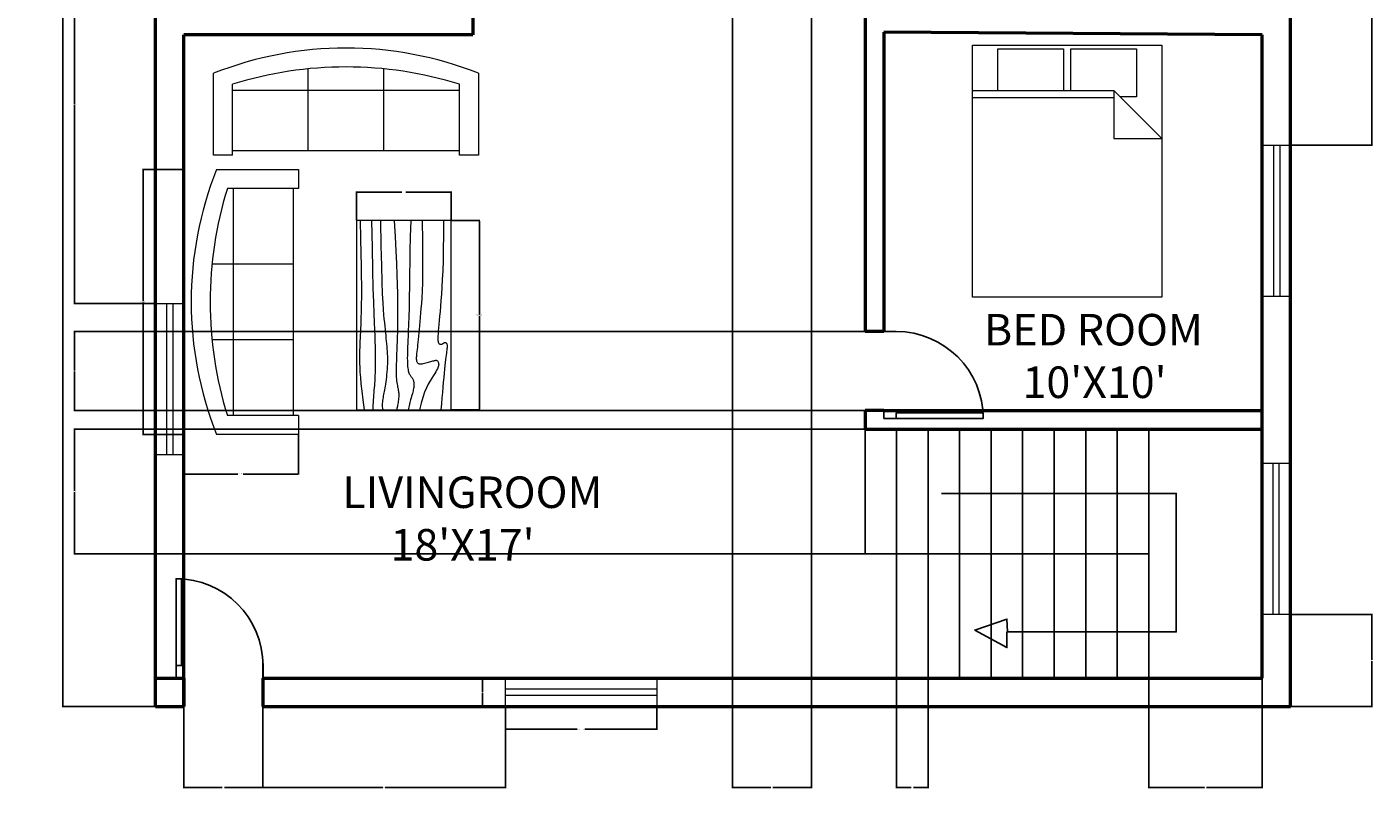
# Model space of a CAD drawing. Units: inches. Extents: x 471 to 898, y -3 to 533.
# Tile 1 of 3: x 471 to 898, y -3 to 239. Entities that reach past the tile are written whole.
import ezdxf

# ---------------------------------------------------------------- set-up
doc = ezdxf.new("R2010")
doc.units = ezdxf.units.IN
doc.header["$MEASUREMENT"] = 0
for name, color, linetype, lineweight in [('A-ANNO-DIMS', 2, 'Continuous', 18), ('A-AREA-IDEN', 7, 'Continuous', 25), ('A-DOOR', 3, 'Continuous', 25), ('A-FLOR-STRS', 7, 'Continuous', 25), ('A-FURN', 8, 'Continuous', 18), ('A-GLAZ', 4, 'Continuous', 18), ('A-WALL', 7, 'Continuous', 50)]:
    doc.layers.add(name, color=color, linetype=linetype, lineweight=lineweight)
doc.styles.get("Standard").update_dxf_attribs({"font": 'arial.ttf'})
doc.dimstyles.get("Standard").update_dxf_attribs({"dimtxt": 0.18, "dimasz": 0.18, "dimexe": 0.18, "dimexo": 0.0625, "dimgap": 0.09, "dimtad": 0, "dimtih": 1, "dimtoh": 1, "dimdec": 1, "dimzin": 0, "dimdsep": 46, "dimlunit": 4, "dimtxsty": 'Standard', "dimcen": 0.09, "dimadec": 0, "dimazin": 0, "dimtfac": 1, "dimtdec": 1, "dimtofl": 0, "dimtmove": 0, "dimatfit": 3, "dimfxl": 1, "dimtolj": 1, "dimtzin": 0, "dimarcsym": 0})

# ---------------------------------------------------------------- blocks, each defined once
blk = doc.blocks.new('Sofa - Roundback 7 ft.')
for p, q in [((-12.00002, -32.4421), (-12.00003, -6.5971)), ((11.99997, -32.4421), (11.99998, -6.5971)), ((-36.000027, -34), (-36.000027, -11.4696)), ((35.99998, -34), (35.99998, -11.4696)), ((-35.999844, -13.3819), (35.9998, -13.3819)), ((-36.000027, -32.4421), (35.99998, -32.4421))]:
    blk.add_line(p, q)
for points in [[(-36.000027, -34), (-42.000027, -34), (-42.000027, -8)], [(41.99998, -8), (41.99998, -34), (35.99998, -34)]]:
    blk.add_lwpolyline(points)
for centre, radius, start, end in [((0, -114.25), 114.25, 68.43141, 111.5686), ((-0.00001, -127.1968), 121.1968, 72.72033, 107.2797)]:
    blk.add_arc(centre, radius, start, end)
blk = doc.blocks.new('Table - Rectangular Woodgrain 60 x 30 in.')
for p, q in [((0, 0), (0, -30)), ((60, 0), (0, 0)), ((60, -30), (60, 0)), ((0, -30), (60, -30))]:
    blk.add_line(p, q)
for points in [[(0, -2.4), (4.8155, -2.418), (9.0302, -2.4688), (12.709, -2.5477), (15.9167, -2.65), (18.7181, -2.7711), (21.1781, -2.9063), (23.3616, -3.0508), (25.3333, -3.2), (27.1477, -3.3495), (28.8172, -3.4958), (30.3437, -3.636), (31.7291, -3.7667), (32.9756, -3.8849), (34.0849, -3.9875), (35.059, -4.0714), (35.9, -4.1334), (36.6114, -4.1711), (37.2041, -4.1854), (37.6906, -4.1779), (38.0833, -4.15), (38.3948, -4.1034), (38.6375, -4.0396), (38.8239, -3.9602), (38.9666, -3.8667), (39.0764, -3.7608), (39.1573, -3.6448), (39.2116, -3.521), (39.2416, -3.3917), (39.2498, -3.2593), (39.2385, -3.1261), (39.21, -2.9944), (39.1666, -2.8667), (39.111, -2.7447), (39.0468, -2.6281), (38.978, -2.5163), (38.9083, -2.4083), (38.8418, -2.3035), (38.7823, -2.201), (38.7337, -2.1001), (38.7, -2), (38.6844, -1.9003), (38.6875, -1.8021), (38.7094, -1.707), (38.75, -1.6167), (38.8094, -1.5326), (38.8875, -1.4563), (38.9844, -1.3893), (39.1, -1.3333), (39.2351, -1.2896), (39.3937, -1.2583), (39.5804, -1.2396), (39.8, -1.2333), (40.057, -1.2396), (40.3562, -1.2583), (40.7023, -1.2896), (41.1, -1.3333), (41.5547, -1.3895), (42.0755, -1.4573), (42.6721, -1.5361), (43.3542, -1.625), (44.1316, -1.7233), (45.014, -1.8302), (46.0114, -1.9449), (47.1333, -2.0667), (48.3862, -2.1947), (49.7625, -2.3281), (51.2513, -2.4663), (52.8416, -2.6083), (54.5226, -2.7535), (56.2833, -2.9011), (58.1127, -3.0501), (60, -3.2)], [(0, -9.2), (6.5759, -9.0858), (11.9385, -9.0365), (16.2527, -9.0418), (19.6833, -9.0917), (22.3952, -9.1759), (24.5531, -9.2844), (26.322, -9.4069), (27.8666, -9.5333), (29.3241, -9.6553), (30.7203, -9.7719), (32.0532, -9.8837), (33.3208, -9.9917), (34.5213, -10.0965), (35.6526, -10.199), (36.7128, -10.2999), (37.7, -10.4), (38.6129, -10.4996), (39.4531, -10.5969), (40.223, -10.6895), (40.925, -10.775), (41.5613, -10.8512), (42.1344, -10.9156), (42.6465, -10.966), (43.1, -11), (43.4976, -11.0158), (43.8437, -11.0136), (44.143, -10.9942), (44.4, -10.9583), (44.6195, -10.9069), (44.8062, -10.8406), (44.9648, -10.7603), (45.1, -10.6667), (45.2155, -10.5598), (45.3114, -10.4365), (45.3871, -10.2929), (45.4416, -10.125), (45.4743, -9.929), (45.4844, -9.7011), (45.4709, -9.4371), (45.4333, -9.1333), (45.3716, -8.7883), (45.2896, -8.4104), (45.1919, -8.0107), (45.0833, -7.6), (44.9685, -7.1893), (44.8521, -6.7896), (44.7388, -6.4117), (44.6333, -6.0667), (44.54, -5.7628), (44.4614, -5.4979), (44.4001, -5.2675), (44.3583, -5.0667), (44.3384, -4.8909), (44.3427, -4.7354), (44.3736, -4.5956), (44.4333, -4.4667), (44.5236, -4.3453), (44.6427, -4.2333), (44.7884, -4.1339), (44.9583, -4.05), (45.1501, -3.9849), (45.3614, -3.9417), (45.59, -3.9234), (45.8333, -3.9333), (46.0915, -3.9749), (46.3734, -4.0531), (46.6906, -4.1736), (47.0542, -4.3417), (47.4756, -4.5629), (47.9661, -4.8427), (48.5372, -5.1866), (49.2, -5.6), (49.9676, -6.0844), (50.8594, -6.625), (51.8965, -7.2031), (53.1, -7.8), (54.491, -8.3969), (56.0906, -8.975), (57.9199, -9.5156), (60, -10)], [(0, -12.8), (5.1847, -12.9322), (9.6213, -13.0323), (13.3963, -13.1059), (16.5958, -13.1583), (19.3063, -13.1952), (21.614, -13.2219), (23.6054, -13.2439), (25.3666, -13.2667), (26.9728, -13.2947), (28.4531, -13.3281), (29.8256, -13.3663), (31.1083, -13.4083), (32.3191, -13.4535), (33.476, -13.501), (34.597, -13.5501), (35.7, -13.6), (36.7984, -13.6497), (37.8875, -13.6979), (38.9578, -13.743), (40, -13.7833), (41.0047, -13.8174), (41.9625, -13.8438), (42.864, -13.8607), (43.7, -13.8667), (44.4631, -13.8604), (45.1552, -13.8417), (45.7801, -13.8104), (46.3416, -13.7667), (46.8439, -13.7104), (47.2906, -13.6417), (47.6858, -13.5604), (48.0333, -13.4667), (48.3375, -13.3608), (48.6042, -13.2448), (48.8396, -13.121), (49.05, -12.9917), (49.2417, -12.8593), (49.4208, -12.7261), (49.5937, -12.5944), (49.7667, -12.4667), (49.9452, -12.3451), (50.1323, -12.2313), (50.3303, -12.1268), (50.5416, -12.0333), (50.7686, -11.9524), (51.0135, -11.8854), (51.2788, -11.8341), (51.5666, -11.8), (51.8785, -11.7843), (52.2116, -11.7865), (52.562, -11.8059), (52.926, -11.8417), (53.2998, -11.8931), (53.6795, -11.9594), (54.0614, -12.0397), (54.4416, -12.1333), (54.8223, -12.2401), (55.2293, -12.3625), (55.6942, -12.5037), (56.2489, -12.6667), (56.9251, -12.8547), (57.7545, -13.0708), (58.7689, -13.3182), (60, -13.6)], [(0, -18), (5.124, -17.7273), (9.6609, -17.5057), (13.6705, -17.3303), (17.2125, -17.1958), (20.3467, -17.0973), (23.1328, -17.0297), (25.6307, -16.9878), (27.9, -16.9667), (29.9928, -16.9617), (31.9302, -16.9703), (33.7254, -16.9907), (35.3917, -17.0208), (36.9423, -17.0588), (38.3906, -17.1026), (39.7499, -17.1503), (41.0333, -17.2), (42.2519, -17.2496), (43.4073, -17.2969), (44.4986, -17.3395), (45.525, -17.375), (46.4858, -17.4012), (47.3802, -17.4156), (48.2074, -17.416), (48.9667, -17.4), (49.6583, -17.3662), (50.2872, -17.3167), (50.8595, -17.2547), (51.3812, -17.1833), (51.8584, -17.1057), (52.2971, -17.025), (52.7034, -16.9443), (53.0833, -16.8667), (53.443, -16.7951), (53.789, -16.7313), (54.128, -16.6768), (54.4666, -16.6334), (54.8115, -16.6024), (55.1693, -16.5854), (55.5465, -16.5841), (55.95, -16.6), (56.3828, -16.6337), (56.8346, -16.6823), (57.2915, -16.7418), (57.7396, -16.8084), (58.165, -16.878), (58.5539, -16.9469), (58.8924, -17.0111), (59.1666, -17.0667), (59.3679, -17.1107), (59.5078, -17.1438), (59.6032, -17.1675), (59.6708, -17.1833), (59.7275, -17.193), (59.7901, -17.1979), (59.8753, -17.1998), (60, -17.2)], [(0, -22.4), (8.0098, -22.2501), (14.4094, -22.1011), (19.4168, -21.9535), (23.25, -21.8083), (26.1269, -21.6663), (28.2656, -21.5281), (29.884, -21.3947), (31.2, -21.2667), (32.3967, -21.1448), (33.5172, -21.0292), (34.5697, -20.9198), (35.5625, -20.8167), (36.5037, -20.7198), (37.4015, -20.6292), (38.2642, -20.5448), (39.1, -20.4667), (39.9164, -20.3951), (40.7187, -20.3313), (41.5117, -20.2768), (42.3, -20.2333), (43.0883, -20.2024), (43.8812, -20.1854), (44.6836, -20.1841), (45.5, -20.2), (46.3328, -20.234), (47.1747, -20.2844), (48.0163, -20.3488), (48.8479, -20.425), (49.66, -20.5106), (50.4429, -20.6031), (51.1872, -20.7004), (51.8833, -20.8), (52.5246, -20.8999), (53.1166, -20.9995), (53.6681, -21.0983), (54.1875, -21.1958), (54.6834, -21.2919), (55.1646, -21.3859), (55.6394, -21.4777), (56.1167, -21.5667), (56.6028, -21.6515), (57.0961, -21.7266), (57.5929, -21.7852), (58.0896, -21.8208), (58.5823, -21.8268), (59.0674, -21.7964), (59.5412, -21.723), (60, -21.6)], [(0, -25.2), (8.6355, -25.0504), (15.7026, -24.9031), (21.4049, -24.7606), (25.9458, -24.625), (29.529, -24.4988), (32.3578, -24.3844), (34.6359, -24.284), (36.5667, -24.2), (38.3213, -24.1341), (39.9417, -24.0854), (41.437, -24.0523), (42.8167, -24.0333), (44.0901, -24.0268), (45.2667, -24.0313), (46.3557, -24.0451), (47.3667, -24.0667), (48.309, -24.0947), (49.1928, -24.1287), (50.0284, -24.168), (50.826, -24.2125), (51.5959, -24.2617), (52.3483, -24.3151), (53.0935, -24.3725), (53.8417, -24.4334), (54.6009, -24.497), (55.3699, -24.561), (56.1454, -24.6226), (56.9239, -24.6792), (57.7021, -24.7279), (58.4764, -24.7662), (59.2435, -24.7911), (60, -24.8)], [(0, -28.8), (5.6867, -28.6681), (10.45, -28.5698), (14.407, -28.5012), (17.675, -28.4584), (20.3711, -28.4374), (22.6125, -28.4344), (24.5164, -28.4455), (26.2, -28.4667), (27.762, -28.4947), (29.2276, -28.5281), (30.6033, -28.5663), (31.8958, -28.6084), (33.1118, -28.6535), (34.2578, -28.7011), (35.3405, -28.7501), (36.3666, -28.8), (37.3443, -28.8497), (38.288, -28.8974), (39.2137, -28.9412), (40.1375, -28.9792), (41.0753, -29.0093), (42.0432, -29.0297), (43.0572, -29.0384), (44.1333, -29.0333), (45.2936, -29.0114), (46.5843, -28.9641), (48.0579, -28.8816), (49.7666, -28.7542), (51.7629, -28.5721), (54.0989, -28.3255), (56.8272, -28.0048), (60, -27.6)]]:
    blk.add_lwpolyline(points)
blk = doc.blocks.new('Bed - Queen')
for p, q in [((0, -80.00003), (0, 0)), ((0, 0), (59.99999, 0)), ((59.99999, 0), (59.99999, -80.00003)), ((7.99999, -1.2), (28.79998, -1.2)), ((7.99999, -14.4), (7.99999, -1.2)), ((28.79998, -1.2), (28.79998, -14.4)), ((31.19999, -1.2), (51.99999, -1.2)), ((31.19999, -14.4), (31.19999, -1.2)), ((51.99999, -1.2), (51.99999, -16.4)), ((0, -14.4), (44.8, -14.4)), ((44.8, -16.8), (0, -16.8)), ((59.99999, -29.6), (44.8, -14.4)), ((44.8, -14.4), (44.8, -29.6)), ((51.99999, -16.4), (46.79936, -16.4)), ((44.8, -29.6), (59.99999, -29.6)), ((59.99999, -80.00003), (0, -80.00003))]:
    blk.add_line(p, q)
blk = doc.blocks.new('*U8')
for p, q in [((0, 0), (0, -100)), ((700, 0), (700, -100))]:
    blk.add_line(p, q)
blk.add_lwpolyline([(0, 0), (0, 700), (43.75, 700), (43.75, 0)], close=True)
blk.add_arc((0, 0), 700, 0, 90)
blk = doc.blocks.new('*D13')
at = {"layer": 'A-ANNO-DIMS', "color": 0, "lineweight": -2, "transparency": 16777216}
for p, q in [((512.17, 503.07), (482.62, 503.07)), ((482.8, 502.89), (482.8, 269.29)), ((482.8, 23.25), (482.8, 256.86)), ((512.17, 23.07), (482.62, 23.07))]:
    blk.add_line(p, q, dxfattribs=at)
at = {"layer": 'A-ANNO-DIMS', "color": 0, "transparency": 16777216}
for points in [[(482.77, 502.89), (482.83, 502.89), (482.8, 503.07)], [(482.77, 23.25), (482.83, 23.25), (482.8, 23.07)]]:
    blk.add_solid(points, dxfattribs=at)
at = {"layer": 'Defpoints', "color": 0, "transparency": 16777216}
for p in [(512.23, 503.07), (482.8, 23.07), (512.23, 23.07)]:
    blk.add_point(p, dxfattribs=at)
at = {"layer": 'A-ANNO-DIMS', "color": 0, "transparency": 16777216, "insert": (482.8, 263.07), "char_height": 12, "attachment_point": 5}
blk.add_mtext("\\A1;40'", dxfattribs=at)
blk = doc.blocks.new('WIN-48X9')
for p, q in [((0, 48), (9, 48)), ((0, 0), (0, 48)), ((3.5, 48), (3.5, 0)), ((5.5, 48), (5.5, 0)), ((9, 48), (9, 0)), ((9, 0), (0, 0))]:
    blk.add_line(p, q)
blk = doc.blocks.new('*D15')
at = {"layer": 'A-ANNO-DIMS', "color": 0, "lineweight": -2, "transparency": 16777216}
for p, q in [((623.17, 23.01), (623.17, 15.69)), ((671.17, 23.01), (671.17, 15.69)), ((623.35, 15.87), (645.94, 15.87)), ((670.99, 15.87), (648.4, 15.87))]:
    blk.add_line(p, q, dxfattribs=at)
at = {"layer": 'A-ANNO-DIMS', "color": 0, "transparency": 16777216}
for points in [[(623.35, 15.9), (623.35, 15.84), (623.17, 15.87)], [(670.99, 15.9), (670.99, 15.84), (671.17, 15.87)]]:
    blk.add_solid(points, dxfattribs=at)
at = {"layer": 'Defpoints', "color": 0, "transparency": 16777216}
for p in [(623.17, 23.07), (671.17, 23.07), (671.17, 15.87)]:
    blk.add_point(p, dxfattribs=at)
at = {"layer": 'A-ANNO-DIMS', "color": 0, "transparency": 16777216, "insert": (647.17, 15.87), "char_height": 0.18, "attachment_point": 5}
blk.add_mtext('\\A1;WINDOW 4\'-0" TYP.', dxfattribs=at)
blk = doc.blocks.new('*D16')
at = {"layer": 'A-ANNO-DIMS', "color": 0, "lineweight": -2, "transparency": 16777216}
for p, q in [((623.11, 32.07), (615.79, 32.07)), ((615.97, 31.89), (615.97, 27.76)), ((615.97, 23.25), (615.97, 27.39)), ((623.11, 23.07), (615.79, 23.07))]:
    blk.add_line(p, q, dxfattribs=at)
at = {"layer": 'A-ANNO-DIMS', "color": 0, "transparency": 16777216}
for points in [[(615.94, 31.89), (616, 31.89), (615.97, 32.07)], [(615.94, 23.25), (616, 23.25), (615.97, 23.07)]]:
    blk.add_solid(points, dxfattribs=at)
at = {"layer": 'Defpoints', "color": 0, "transparency": 16777216}
for p in [(623.17, 32.07), (615.97, 23.07), (623.17, 23.07)]:
    blk.add_point(p, dxfattribs=at)
at = {"layer": 'A-ANNO-DIMS', "color": 0, "transparency": 16777216, "insert": (615.97, 27.57), "char_height": 0.18, "attachment_point": 5}
blk.add_mtext('\\A1;0\'-9" TYP.', dxfattribs=at)
blk = doc.blocks.new('*D19')
at = {"layer": 'A-ANNO-DIMS', "color": 0, "lineweight": -2, "transparency": 16777216}
for p, q in [((606.01, 177.21), (615.13, 177.21)), ((614.95, 177.03), (614.95, 147.39)), ((614.95, 117.39), (614.95, 147.03)), ((606.01, 117.21), (615.13, 117.21))]:
    blk.add_line(p, q, dxfattribs=at)
at = {"layer": 'A-ANNO-DIMS', "color": 0, "transparency": 16777216}
for points in [[(614.92, 177.03), (614.98, 177.03), (614.95, 177.21)], [(614.92, 117.39), (614.98, 117.39), (614.95, 117.21)]]:
    blk.add_solid(points, dxfattribs=at)
at = {"layer": 'Defpoints', "color": 0, "transparency": 16777216}
for p in [(605.95, 177.21), (605.95, 117.21), (614.95, 117.21)]:
    blk.add_point(p, dxfattribs=at)
at = {"layer": 'A-ANNO-DIMS', "color": 0, "transparency": 16777216, "insert": (614.95, 147.21), "char_height": 0.18, "attachment_point": 5}
blk.add_mtext('\\A1;TABLE 5\'-0" TYP.', dxfattribs=at)
blk = doc.blocks.new('*D20')
at = {"layer": 'A-ANNO-DIMS', "color": 0, "lineweight": -2, "transparency": 16777216}
for p, q in [((575.95, 177.28), (575.95, 186.39)), ((576.13, 186.21), (590.31, 186.21)), ((605.77, 186.21), (591.59, 186.21)), ((605.95, 177.28), (605.95, 186.39))]:
    blk.add_line(p, q, dxfattribs=at)
at = {"layer": 'A-ANNO-DIMS', "color": 0, "transparency": 16777216}
for points in [[(576.13, 186.24), (576.13, 186.18), (575.95, 186.21)], [(605.77, 186.24), (605.77, 186.18), (605.95, 186.21)]]:
    blk.add_solid(points, dxfattribs=at)
at = {"layer": 'Defpoints', "color": 0, "transparency": 16777216}
for p in [(605.95, 186.21), (575.95, 177.21), (605.95, 177.21)]:
    blk.add_point(p, dxfattribs=at)
at = {"layer": 'A-ANNO-DIMS', "color": 0, "transparency": 16777216, "insert": (590.95, 186.21), "char_height": 0.18, "attachment_point": 5}
blk.add_mtext('\\A1;2\'-6" TYP.', dxfattribs=at)
blk = doc.blocks.new('*D21')
at = {"layer": 'A-ANNO-DIMS', "color": 0, "lineweight": -2, "transparency": 16777216}
for p, q in [((520.81, 193.39), (508.09, 193.39)), ((508.27, 193.21), (508.27, 151.58)), ((508.27, 109.57), (508.27, 151.21)), ((520.81, 109.39), (508.09, 109.39))]:
    blk.add_line(p, q, dxfattribs=at)
at = {"layer": 'A-ANNO-DIMS', "color": 0, "transparency": 16777216}
for points in [[(508.24, 193.21), (508.3, 193.21), (508.27, 193.39)], [(508.24, 109.57), (508.3, 109.57), (508.27, 109.39)]]:
    blk.add_solid(points, dxfattribs=at)
at = {"layer": 'Defpoints', "color": 0, "transparency": 16777216}
for p in [(508.27, 193.39), (520.87, 193.39), (520.87, 109.39)]:
    blk.add_point(p, dxfattribs=at)
at = {"layer": 'A-ANNO-DIMS', "color": 0, "transparency": 16777216, "insert": (508.27, 151.39), "char_height": 0.18, "attachment_point": 5}
blk.add_mtext('\\A1;SOFA 7\'-0" TYP.', dxfattribs=at)
blk = doc.blocks.new('*D22')
at = {"layer": 'A-ANNO-DIMS', "color": 0, "lineweight": -2, "transparency": 16777216}
for p, q in [((520.87, 109.33), (520.87, 96.61)), ((557.54, 109.33), (557.54, 96.61)), ((521.05, 96.79), (538.36, 96.79)), ((557.36, 96.79), (540.05, 96.79))]:
    blk.add_line(p, q, dxfattribs=at)
at = {"layer": 'A-ANNO-DIMS', "color": 0, "transparency": 16777216}
for points in [[(521.05, 96.82), (521.05, 96.76), (520.87, 96.79)], [(557.36, 96.82), (557.36, 96.76), (557.54, 96.79)]]:
    blk.add_solid(points, dxfattribs=at)
at = {"layer": 'Defpoints', "color": 0, "transparency": 16777216}
for p in [(520.87, 109.39), (557.54, 109.39), (520.87, 96.79)]:
    blk.add_point(p, dxfattribs=at)
at = {"layer": 'A-ANNO-DIMS', "color": 0, "transparency": 16777216, "insert": (539.21, 96.79), "char_height": 0.18, "attachment_point": 5}
blk.add_mtext('\\A1;3\'-0 1/2" TYP.', dxfattribs=at)
blk = doc.blocks.new('*D33')
at = {"layer": 'A-ANNO-DIMS', "color": 0, "lineweight": -2, "transparency": 16777216}
for p, q in [((521.23, 23.01), (521.23, -2.81)), ((546.23, 23.01), (546.23, -2.81)), ((521.41, -2.63), (533.4, -2.63)), ((546.05, -2.63), (534.06, -2.63))]:
    blk.add_line(p, q, dxfattribs=at)
at = {"layer": 'A-ANNO-DIMS', "color": 0, "transparency": 16777216}
for points in [[(521.41, -2.6), (521.41, -2.66), (521.23, -2.63)], [(546.05, -2.6), (546.05, -2.66), (546.23, -2.63)]]:
    blk.add_solid(points, dxfattribs=at)
at = {"layer": 'Defpoints', "color": 0, "transparency": 16777216}
for p in [(521.23, 23.07), (546.23, 23.07), (546.23, -2.63)]:
    blk.add_point(p, dxfattribs=at)
at = {"layer": 'A-ANNO-DIMS', "color": 0, "transparency": 16777216, "insert": (533.73, -2.63), "char_height": 0.18, "attachment_point": 5}
blk.add_mtext('\\A1;2\'-1"', dxfattribs=at)
blk = doc.blocks.new('*D34')
at = {"layer": 'A-ANNO-DIMS', "color": 0, "lineweight": -2, "transparency": 16777216}
for p, q in [((546.23, 23.01), (546.23, -2.81)), ((623.17, 23.01), (623.17, -2.81)), ((546.41, -2.63), (584.37, -2.63)), ((622.99, -2.63), (585.03, -2.63))]:
    blk.add_line(p, q, dxfattribs=at)
at = {"layer": 'A-ANNO-DIMS', "color": 0, "transparency": 16777216}
for points in [[(546.41, -2.6), (546.41, -2.66), (546.23, -2.63)], [(622.99, -2.6), (622.99, -2.66), (623.17, -2.63)]]:
    blk.add_solid(points, dxfattribs=at)
at = {"layer": 'Defpoints', "color": 0, "transparency": 16777216}
for p in [(546.23, 23.07), (623.17, 23.07), (623.17, -2.63)]:
    blk.add_point(p, dxfattribs=at)
at = {"layer": 'A-ANNO-DIMS', "color": 0, "transparency": 16777216, "insert": (584.7, -2.63), "char_height": 0.18, "attachment_point": 5}
blk.add_mtext('\\A1;6\'-5"', dxfattribs=at)
blk = doc.blocks.new('*D37')
at = {"layer": 'A-ANNO-DIMS', "color": 0, "lineweight": -2, "transparency": 16777216}
for p, q in [((512.17, 277.18), (486.35, 277.18)), ((486.53, 277), (486.53, 214.23)), ((486.53, 151.09), (486.53, 213.86)), ((512.17, 150.91), (486.35, 150.91))]:
    blk.add_line(p, q, dxfattribs=at)
at = {"layer": 'A-ANNO-DIMS', "color": 0, "transparency": 16777216}
for points in [[(486.5, 277), (486.56, 277), (486.53, 277.18)], [(486.5, 151.09), (486.56, 151.09), (486.53, 150.91)]]:
    blk.add_solid(points, dxfattribs=at)
at = {"layer": 'Defpoints', "color": 0, "transparency": 16777216}
for p in [(512.23, 277.18), (486.53, 150.91), (512.23, 150.91)]:
    blk.add_point(p, dxfattribs=at)
at = {"layer": 'A-ANNO-DIMS', "color": 0, "transparency": 16777216, "insert": (486.53, 214.04), "char_height": 0.18, "attachment_point": 5}
blk.add_mtext('\\A1;10\'-6 1/2"', dxfattribs=at)
blk = doc.blocks.new('*D40')
at = {"layer": 'A-ANNO-DIMS', "color": 0, "lineweight": -2, "transparency": 16777216}
for p, q in [((872.29, 380.09), (898.15, 380.09)), ((897.97, 379.91), (897.97, 290.77)), ((897.97, 201.27), (897.97, 290.41)), ((872.33, 201.09), (898.15, 201.09))]:
    blk.add_line(p, q, dxfattribs=at)
at = {"layer": 'A-ANNO-DIMS', "color": 0, "transparency": 16777216}
for points in [[(897.94, 379.91), (898, 379.91), (897.97, 380.09)], [(897.94, 201.27), (898, 201.27), (897.97, 201.09)]]:
    blk.add_solid(points, dxfattribs=at)
at = {"layer": 'Defpoints', "color": 0, "transparency": 16777216}
for p in [(872.23, 380.09), (872.27, 201.09), (897.97, 201.09)]:
    blk.add_point(p, dxfattribs=at)
at = {"layer": 'A-ANNO-DIMS', "color": 0, "transparency": 16777216, "insert": (897.97, 290.59), "char_height": 0.18, "attachment_point": 5}
blk.add_mtext('\\A1;14\'-11"', dxfattribs=at)
blk = doc.blocks.new('*D41')
at = {"layer": 'A-ANNO-DIMS', "color": 0, "lineweight": -2, "transparency": 16777216}
for p, q in [((872.1, 52.21), (898.15, 52.21)), ((897.97, 52.03), (897.97, 37.83)), ((897.97, 23.25), (897.97, 37.46)), ((872.29, 23.07), (898.15, 23.07))]:
    blk.add_line(p, q, dxfattribs=at)
at = {"layer": 'A-ANNO-DIMS', "color": 0, "transparency": 16777216}
for points in [[(897.94, 52.03), (898, 52.03), (897.97, 52.21)], [(897.94, 23.25), (898, 23.25), (897.97, 23.07)]]:
    blk.add_solid(points, dxfattribs=at)
at = {"layer": 'Defpoints', "color": 0, "transparency": 16777216}
for p in [(872.04, 52.21), (897.97, 52.21), (872.23, 23.07)]:
    blk.add_point(p, dxfattribs=at)
at = {"layer": 'A-ANNO-DIMS', "color": 0, "transparency": 16777216, "insert": (897.97, 37.64), "char_height": 0.18, "attachment_point": 5}
blk.add_mtext('\\A1;2\'-5"', dxfattribs=at)
blk = doc.blocks.new('*D42')
at = {"layer": 'A-ANNO-DIMS', "color": 0, "lineweight": -2, "transparency": 16777216}
for p, q in [((737.17, 111), (486.35, 111)), ((486.53, 110.82), (486.53, 91.45)), ((486.53, 71.72), (486.53, 91.09)), ((737.17, 71.54), (486.35, 71.54))]:
    blk.add_line(p, q, dxfattribs=at)
at = {"layer": 'A-ANNO-DIMS', "color": 0, "transparency": 16777216}
for points in [[(486.5, 110.82), (486.56, 110.82), (486.53, 111)], [(486.5, 71.72), (486.56, 71.72), (486.53, 71.54)]]:
    blk.add_solid(points, dxfattribs=at)
at = {"layer": 'Defpoints', "color": 0, "transparency": 16777216}
for p in [(486.53, 111), (737.24, 111), (737.24, 71.54)]:
    blk.add_point(p, dxfattribs=at)
at = {"layer": 'A-ANNO-DIMS', "color": 0, "transparency": 16777216, "insert": (486.53, 91.27), "char_height": 0.18, "attachment_point": 5}
blk.add_mtext('\\A1;3\'-3 1/2"', dxfattribs=at)
blk = doc.blocks.new('*D43')
at = {"layer": 'A-ANNO-DIMS', "color": 0, "lineweight": -2, "transparency": 16777216}
for p, q in [((827.24, 32.01), (827.24, -2.81)), ((863.23, 32.01), (863.23, -2.81)), ((827.42, -2.63), (844.9, -2.63)), ((863.05, -2.63), (845.56, -2.63))]:
    blk.add_line(p, q, dxfattribs=at)
at = {"layer": 'A-ANNO-DIMS', "color": 0, "transparency": 16777216}
for points in [[(827.42, -2.6), (827.42, -2.66), (827.24, -2.63)], [(863.05, -2.6), (863.05, -2.66), (863.23, -2.63)]]:
    blk.add_solid(points, dxfattribs=at)
at = {"layer": 'Defpoints', "color": 0, "transparency": 16777216}
for p in [(827.24, 32.07), (863.23, 32.07), (863.23, -2.63)]:
    blk.add_point(p, dxfattribs=at)
at = {"layer": 'A-ANNO-DIMS', "color": 0, "transparency": 16777216, "insert": (845.23, -2.63), "char_height": 0.18, "attachment_point": 5}
blk.add_mtext('\\A1;3\'-0"', dxfattribs=at)
blk = doc.blocks.new('*D46')
at = {"layer": 'A-ANNO-DIMS', "color": 0, "lineweight": -2, "transparency": 16777216}
for p, q in [((747.24, 32.01), (747.24, -2.81)), ((757.24, 32.01), (757.24, -2.81)), ((747.42, -2.63), (751.84, -2.63)), ((757.06, -2.63), (752.63, -2.63))]:
    blk.add_line(p, q, dxfattribs=at)
at = {"layer": 'A-ANNO-DIMS', "color": 0, "transparency": 16777216}
for points in [[(747.42, -2.6), (747.42, -2.66), (747.24, -2.63)], [(757.06, -2.6), (757.06, -2.66), (757.24, -2.63)]]:
    blk.add_solid(points, dxfattribs=at)
at = {"layer": 'Defpoints', "color": 0, "transparency": 16777216}
for p in [(747.24, 32.07), (757.24, 32.07), (757.24, -2.63)]:
    blk.add_point(p, dxfattribs=at)
at = {"layer": 'A-ANNO-DIMS', "color": 0, "transparency": 16777216, "insert": (752.24, -2.63), "char_height": 0.18, "attachment_point": 5}
blk.add_mtext('\\A1;0\'-10"', dxfattribs=at)
blk = doc.blocks.new('*D48')
at = {"layer": 'A-ANNO-DIMS', "color": 0, "lineweight": -2, "transparency": 16777216}
for p, q in [((695.23, 314.01), (695.23, -2.81)), ((720.23, 314.01), (720.23, -2.81)), ((695.41, -2.63), (707.4, -2.63)), ((720.05, -2.63), (708.06, -2.63))]:
    blk.add_line(p, q, dxfattribs=at)
at = {"layer": 'A-ANNO-DIMS', "color": 0, "transparency": 16777216}
for points in [[(695.41, -2.6), (695.41, -2.66), (695.23, -2.63)], [(720.05, -2.6), (720.05, -2.66), (720.23, -2.63)]]:
    blk.add_solid(points, dxfattribs=at)
at = {"layer": 'Defpoints', "color": 0, "transparency": 16777216}
for p in [(695.23, 314.07), (720.23, 314.07), (720.23, -2.63)]:
    blk.add_point(p, dxfattribs=at)
at = {"layer": 'A-ANNO-DIMS', "color": 0, "transparency": 16777216, "insert": (707.73, -2.63), "char_height": 0.18, "attachment_point": 5}
blk.add_mtext('\\A1;2\'-1"', dxfattribs=at)
blk = doc.blocks.new('*D49')
at = {"layer": 'A-ANNO-DIMS', "color": 0, "lineweight": -2, "transparency": 16777216}
for p, q in [((737.17, 142), (486.35, 142)), ((486.53, 141.82), (486.53, 129.68)), ((486.53, 117.18), (486.53, 129.32)), ((737.17, 117), (486.35, 117))]:
    blk.add_line(p, q, dxfattribs=at)
at = {"layer": 'A-ANNO-DIMS', "color": 0, "transparency": 16777216}
for points in [[(486.5, 141.82), (486.56, 141.82), (486.53, 142)], [(486.5, 117.18), (486.56, 117.18), (486.53, 117)]]:
    blk.add_solid(points, dxfattribs=at)
at = {"layer": 'Defpoints', "color": 0, "transparency": 16777216}
for p in [(486.53, 142), (737.24, 142), (737.24, 117)]:
    blk.add_point(p, dxfattribs=at)
at = {"layer": 'A-ANNO-DIMS', "color": 0, "transparency": 16777216, "insert": (486.53, 129.5), "char_height": 0.18, "attachment_point": 5}
blk.add_mtext('\\A1;2\'-1"', dxfattribs=at)

msp = doc.modelspace()

# ---------------------------------------------------------------- linework, layer by layer
at = {"layer": 'A-DOOR'}
for p, q in [((743.24, 117.21), (743.24, 117)), ((743.24, 114.44), (743.24, 117)), ((521.23, 38.07), (521.23, 32.07)), ((546.23, 38.07), (546.23, 32.07)), ((518.76, 32.12), (521.23, 32.07))]:
    msp.add_line(p, q, dxfattribs=at)
at = {"layer": 'A-FLOR-STRS'}
for p, q in [((737.24, 111), (737.24, 71.54)), ((747.24, 111), (747.24, 32.07)), ((757.24, 111), (757.24, 32.07)), ((767.24, 111), (767.24, 32.07)), ((777.24, 111), (777.24, 32.07)), ((787.24, 111), (787.24, 32.07)), ((797.24, 111), (797.24, 32.07)), ((807.24, 111), (807.24, 32.07)), ((817.24, 111), (817.24, 32.07)), ((827.24, 111), (827.24, 32.07)), ((737.24, 71.54), (827.24, 71.54))]:
    msp.add_line(p, q, dxfattribs=at)
msp.add_lwpolyline([(761.52, 90.66), (835.95, 90.66), (835.95, 46.7), (782.23, 46.7), (782.23, 41.74), (772.04, 47.32), (782.24, 50.82), (782.4, 46.7)], dxfattribs=at)
at = {"layer": 'A-WALL'}
for p, q in [((512.23, 23.07), (512.23, 503.07)), ((872.23, 23.07), (872.23, 503.07)), ((612.83, 242.07), (612.83, 236.07)), ((737.24, 243.05), (737.24, 142)), ((521.23, 23.07), (521.23, 236.07)), ((612.83, 236.07), (521.23, 236.07)), ((863.23, 236.07), (743.24, 237)), ((743.24, 237), (743.24, 142)), ((863.23, 32.07), (863.23, 236.07)), ((743.24, 142), (737.24, 142)), ((743.24, 117), (737.24, 117)), ((737.24, 117), (737.24, 111)), ((743.24, 117), (863.24, 117)), ((737.24, 111), (863.24, 111)), ((512.23, 32.07), (521.23, 32.07)), ((521.23, 32.07), (521.23, 23.07)), ((546.23, 32.07), (863.23, 32.07)), ((546.23, 32.07), (546.23, 23.07)), ((872.04, 32.07), (872.23, 32.07)), ((512.23, 23.07), (521.23, 23.07)), ((546.23, 23.07), (872.23, 23.07))]:
    msp.add_line(p, q, dxfattribs=at)

# ---------------------------------------------------------------- block references
at = {"layer": 'A-DOOR', "xscale": -0.0393700787401575, "yscale": 0.0393700787401575, "zscale": 0.0393700787401575, "rotation": 270}
msp.add_blockref('*U8', (747.17, 114.44), dxfattribs=at)
at = {"layer": 'A-DOOR', "xscale": 0.0393700787401575, "yscale": 0.0393700787401575, "zscale": 0.0393700787401575}
msp.add_blockref('*U8', (518.76, 36.05), dxfattribs=at)
at = {"layer": 'A-FURN'}
for name, p in [('Sofa - Roundback 7 ft.', (572.66, 231.91)), ('Bed - Queen', (771.35, 232.87))]:
    msp.add_blockref(name, p, dxfattribs=at)
for name, p, rotation in [('Sofa - Roundback 7 ft.', (523.54, 151.39), 90), ('Table - Rectangular Woodgrain 60 x 30 in.', (605.95, 177.21), 270)]:
    msp.add_blockref(name, p, dxfattribs=dict(at, rotation=rotation))
at = {"layer": 'A-GLAZ'}
for p in [(863.27, 153.09), (512.23, 102.91), (863.04, 52.21)]:
    msp.add_blockref('WIN-48X9', p, dxfattribs=at)
at = {"layer": 'A-GLAZ', "rotation": 269.9999999999995}
msp.add_blockref('WIN-48X9', (623.17, 32.07), dxfattribs=at)

# ---------------------------------------------------------------- texts
at = {"layer": 'A-AREA-IDEN', "char_height": 10, "attachment_point": 1}
for s, insert in [("BED ROOM \\P    10'X10'", (774.97, 147.58)), ("LIVINGROOM\\P     18'X17'", (571.47, 96.03))]:
    msp.add_mtext_dynamic_manual_height_columns(s, width=80.8054, gutter_width=1, heights=[0], dxfattribs=dict(at, insert=insert))

# ---------------------------------------------------------------- dimensions: what is measured, and where the dimension line sits
at = {"layer": 'A-ANNO-DIMS'}
for base, p1, p2, override, picture, middle in [((482.8, 23.07), (512.23, 503.07), (512.23, 23.07), {"dimtxt": 12, "dimclrd": 0, "dimclre": 0, "dimclrt": 0}, '*D13', (482.8, 263.07)), ((897.97, 201.09), (872.23, 380.09), (872.27, 201.09), {"dimdec": 1, "dimlfac": 1, "dimrnd": 0, "dimzin": 1, "dimdsep": 46, "dimlunit": 4, "dimfrac": 2}, '*D40', (897.97, 290.59)), ((486.53, 150.91), (512.23, 277.18), (512.23, 150.91), {"dimdec": 1, "dimlfac": 1, "dimrnd": 0, "dimzin": 1, "dimdsep": 46, "dimlunit": 4, "dimfrac": 2}, '*D37', (486.53, 214.04)), ((486.53, 142), (737.24, 117), (737.24, 142), {"dimdec": 1, "dimlfac": 1, "dimrnd": 0, "dimzin": 1, "dimdsep": 46, "dimlunit": 4, "dimfrac": 2}, '*D49', (486.53, 129.5)), ((486.53, 111), (737.24, 71.54), (737.24, 111), {"dimdec": 1, "dimlfac": 1, "dimrnd": 0, "dimzin": 1, "dimdsep": 46, "dimlunit": 4, "dimfrac": 2}, '*D42', (486.53, 91.27)), ((897.97, 52.21), (872.23, 23.07), (872.04, 52.21), {"dimdec": 1, "dimlfac": 1, "dimrnd": 0, "dimzin": 1, "dimdsep": 46, "dimlunit": 4, "dimfrac": 2}, '*D41', (897.97, 37.64))]:
    dim = msp.add_linear_dim(base=base, p1=p1, p2=p2, angle=90, dimstyle='Standard', override=override, dxfattribs=at)
    dim.commit()
    dim.dimension.update_dxf_attribs({"geometry": picture, "text_midpoint": middle})
for base, p1, p2, picture, middle in [((720.23, -2.63), (695.23, 314.07), (720.23, 314.07), '*D48', (707.73, -2.63)), ((757.24, -2.63), (747.24, 32.07), (757.24, 32.07), '*D46', (752.24, -2.63)), ((863.23, -2.63), (827.24, 32.07), (863.23, 32.07), '*D43', (845.23, -2.63)), ((546.23, -2.63), (521.23, 23.07), (546.23, 23.07), '*D33', (533.73, -2.63)), ((623.17, -2.63), (546.23, 23.07), (623.17, 23.07), '*D34', (584.7, -2.63))]:
    dim = msp.add_linear_dim(base=base, p1=p1, p2=p2, dimstyle='Standard', override={"dimdec": 1, "dimlfac": 1, "dimrnd": 0, "dimzin": 1, "dimdsep": 46, "dimlunit": 4, "dimfrac": 2}, dxfattribs=at)
    dim.commit()
    dim.dimension.update_dxf_attribs({"geometry": picture, "text_midpoint": middle})
for base, p1, p2, angle, text, picture, middle in [((508.27, 193.39), (520.87, 109.39), (520.87, 193.39), 90, 'SOFA <> TYP.', '*D21', (508.27, 151.39)), ((614.95, 117.21), (605.95, 177.21), (605.95, 117.21), 270, 'TABLE <> TYP.', '*D19', (614.95, 147.21)), ((520.87, 96.79), (557.54, 109.39), (520.87, 109.39), 180, '<> TYP.', '*D22', (539.21, 96.79)), ((615.97, 23.07), (623.17, 32.07), (623.17, 23.07), 270, '<> TYP.', '*D16', (615.97, 27.57))]:
    dim = msp.add_linear_dim(base=base, p1=p1, p2=p2, angle=angle, text=text, dimstyle='Standard', override={"dimdec": 1, "dimlfac": 1, "dimrnd": 0, "dimzin": 1, "dimdsep": 46, "dimlunit": 4, "dimfrac": 2}, dxfattribs=at)
    dim.commit()
    dim.dimension.update_dxf_attribs({"geometry": picture, "text_midpoint": middle})
for base, p1, p2, text, picture, middle in [((605.95, 186.21), (575.95, 177.21), (605.95, 177.21), '<> TYP.', '*D20', (590.95, 186.21)), ((671.17, 15.87), (623.17, 23.07), (671.17, 23.07), 'WINDOW <> TYP.', '*D15', (647.17, 15.87))]:
    dim = msp.add_linear_dim(base=base, p1=p1, p2=p2, text=text, dimstyle='Standard', override={"dimdec": 1, "dimlfac": 1, "dimrnd": 0, "dimzin": 1, "dimdsep": 46, "dimlunit": 4, "dimfrac": 2}, dxfattribs=at)
    dim.commit()
    dim.dimension.update_dxf_attribs({"geometry": picture, "text_midpoint": middle})

doc.saveas('drawing.dxf')
